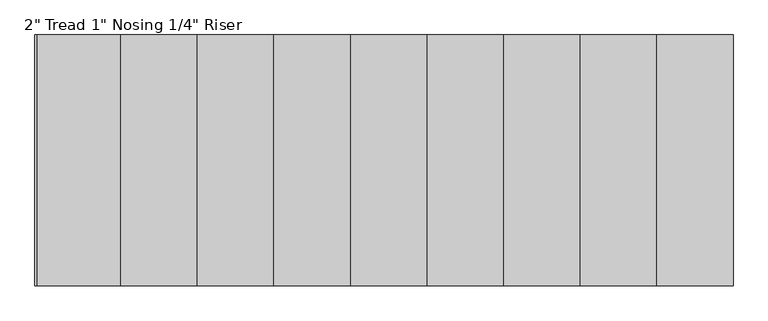
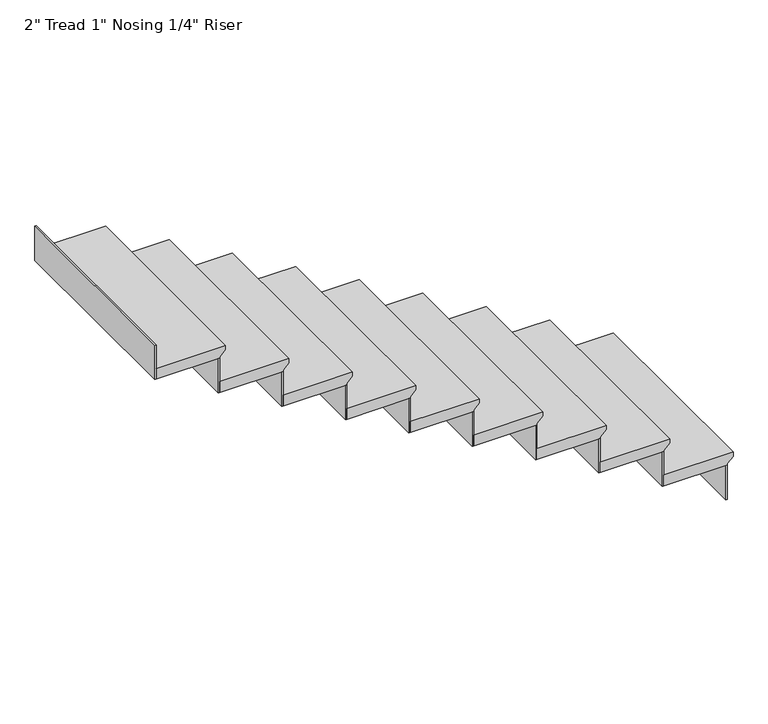
"""IFC4 building model written with IfcOpenShell, lengths in millimetres: stair flight geometry."""

from ifc_helpers import new_model, si_unit, frame, origin, place, context, project, spatial, polyline, outline, extrude, source, transform, mapped, element, save


def stair_flight_043378c7(model_context):
    return source(origin(), model_context, "Body", "SweptSolid", [
        extrude(outline(polyline([(4960.62, 923.4845537), (4960.62, 618.6845537), (4909.82, 618.6845537), (4909.82, 898.0845537), (4916.17, 898.0845537), (4941.57, 923.4845537), (4960.62, 923.4845537)])), frame((0.0, -5753.3544725, 0.0), z_axis=(0.0, 1.0, 0.0), x_axis=(0.0, 0.0, 1.0)), (0.0, 0.0, 1.0), 914.4),
        extrude(outline(polyline([(891.7345537, -4838.9544725), (898.0845537, -4838.9544725), (898.0845537, -5753.3544725), (891.7345537, -5753.3544725), (891.7345537, -4838.9544725)])), frame((0.0, 0.0, 4749.8), z_axis=(0.0, 0.0, 1.0), x_axis=(1.0, 0.0, 0.0)), (0.0, 0.0, 1.0), 160.02),
        extrude(outline(polyline([(612.3345537, -4838.9544725), (618.6845537, -4838.9544725), (618.6845537, -5753.3544725), (612.3345537, -5753.3544725), (612.3345537, -4838.9544725)])), frame((0.0, 0.0, 4909.82), z_axis=(0.0, 0.0, 1.0), x_axis=(1.0, 0.0, 0.0)), (0.0, 0.0, 1.0), 160.02),
        extrude(outline(polyline([(5120.64, 644.0845537), (5120.64, 339.2845537), (5069.84, 339.2845537), (5069.84, 618.6845537), (5076.19, 618.6845537), (5101.59, 644.0845537), (5120.64, 644.0845537)])), frame((0.0, -5753.3544725, 0.0), z_axis=(0.0, 1.0, 0.0), x_axis=(0.0, 0.0, 1.0)), (0.0, 0.0, 1.0), 914.4),
        extrude(outline(polyline([(332.9345537, -4838.9544725), (339.2845537, -4838.9544725), (339.2845537, -5753.3544725), (332.9345537, -5753.3544725), (332.9345537, -4838.9544725)])), frame((0.0, 0.0, 5069.84), z_axis=(0.0, 0.0, 1.0), x_axis=(1.0, 0.0, 0.0)), (0.0, 0.0, 1.0), 160.02),
        extrude(outline(polyline([(5280.66, 364.6845537), (5280.66, 59.8845537), (5229.86, 59.8845537), (5229.86, 339.2845537), (5236.21, 339.2845537), (5261.61, 364.6845537), (5280.66, 364.6845537)])), frame((0.0, -5753.3544725, 0.0), z_axis=(0.0, 1.0, 0.0), x_axis=(0.0, 0.0, 1.0)), (0.0, 0.0, 1.0), 914.4),
        extrude(outline(polyline([(53.5345537, -4838.9544725), (59.8845537, -4838.9544725), (59.8845537, -5753.3544725), (53.5345537, -5753.3544725), (53.5345537, -4838.9544725)])), frame((0.0, 0.0, 5229.86), z_axis=(0.0, 0.0, 1.0), x_axis=(1.0, 0.0, 0.0)), (0.0, 0.0, 1.0), 160.02),
        extrude(outline(polyline([(5440.68, 85.2845537), (5440.68, -219.5154463), (5389.88, -219.5154463), (5389.88, 59.8845537), (5396.23, 59.8845537), (5421.63, 85.2845537), (5440.68, 85.2845537)])), frame((0.0, -5753.3544725, 0.0), z_axis=(0.0, 1.0, 0.0), x_axis=(0.0, 0.0, 1.0)), (0.0, 0.0, 1.0), 914.4),
        extrude(outline(polyline([(-225.8654463, -4838.9544725), (-219.5154463, -4838.9544725), (-219.5154463, -5753.3544725), (-225.8654463, -5753.3544725), (-225.8654463, -4838.9544725)])), frame((0.0, 0.0, 5389.88), z_axis=(0.0, 0.0, 1.0), x_axis=(1.0, 0.0, 0.0)), (0.0, 0.0, 1.0), 160.02),
        extrude(outline(polyline([(5600.7, -194.1154463), (5600.7, -498.9154463), (5549.9, -498.9154463), (5549.9, -219.5154463), (5556.25, -219.5154463), (5581.65, -194.1154463), (5600.7, -194.1154463)])), frame((0.0, -5753.3544725, 0.0), z_axis=(0.0, 1.0, 0.0), x_axis=(0.0, 0.0, 1.0)), (0.0, 0.0, 1.0), 914.4),
        extrude(outline(polyline([(-505.2654463, -4838.9544725), (-498.9154463, -4838.9544725), (-498.9154463, -5753.3544725), (-505.2654463, -5753.3544725), (-505.2654463, -4838.9544725)])), frame((0.0, 0.0, 5549.9), z_axis=(0.0, 0.0, 1.0), x_axis=(1.0, 0.0, 0.0)), (0.0, 0.0, 1.0), 160.02),
        extrude(outline(polyline([(5760.72, -473.5154463), (5760.72, -778.3154463), (5709.92, -778.3154463), (5709.92, -498.9154463), (5716.27, -498.9154463), (5741.67, -473.5154463), (5760.72, -473.5154463)])), frame((0.0, -5753.3544725, 0.0), z_axis=(0.0, 1.0, 0.0), x_axis=(0.0, 0.0, 1.0)), (0.0, 0.0, 1.0), 914.4),
        extrude(outline(polyline([(-784.6654463, -4838.9544725), (-778.3154463, -4838.9544725), (-778.3154463, -5753.3544725), (-784.6654463, -5753.3544725), (-784.6654463, -4838.9544725)])), frame((0.0, 0.0, 5709.92), z_axis=(0.0, 0.0, 1.0), x_axis=(1.0, 0.0, 0.0)), (0.0, 0.0, 1.0), 160.02),
        extrude(outline(polyline([(5920.74, -752.9154463), (5920.74, -1057.7154463), (5869.94, -1057.7154463), (5869.94, -778.3154463), (5876.29, -778.3154463), (5901.69, -752.9154463), (5920.74, -752.9154463)])), frame((0.0, -5753.3544725, 0.0), z_axis=(0.0, 1.0, 0.0), x_axis=(0.0, 0.0, 1.0)), (0.0, 0.0, 1.0), 914.4),
        extrude(outline(polyline([(-1064.0654463, -4838.9544725), (-1057.7154463, -4838.9544725), (-1057.7154463, -5753.3544725), (-1064.0654463, -5753.3544725), (-1064.0654463, -4838.9544725)])), frame((0.0, 0.0, 5869.94), z_axis=(0.0, 0.0, 1.0), x_axis=(1.0, 0.0, 0.0)), (0.0, 0.0, 1.0), 160.02),
        extrude(outline(polyline([(6080.76, -1032.3154463), (6080.76, -1337.1154463), (6029.96, -1337.1154463), (6029.96, -1057.7154463), (6036.31, -1057.7154463), (6061.71, -1032.3154463), (6080.76, -1032.3154463)])), frame((0.0, -5753.3544725, 0.0), z_axis=(0.0, 1.0, 0.0), x_axis=(0.0, 0.0, 1.0)), (0.0, 0.0, 1.0), 914.4),
        extrude(outline(polyline([(-1343.4654463, -4838.9544725), (-1337.1154463, -4838.9544725), (-1337.1154463, -5753.3544725), (-1343.4654463, -5753.3544725), (-1343.4654463, -4838.9544725)])), frame((0.0, 0.0, 6029.96), z_axis=(0.0, 0.0, 1.0), x_axis=(1.0, 0.0, 0.0)), (0.0, 0.0, 1.0), 160.02),
        extrude(outline(polyline([(-1622.8654463, -4838.9544725), (-1616.5154463, -4838.9544725), (-1616.5154463, -5753.3544725), (-1622.8654463, -5753.3544725), (-1622.8654463, -4838.9544725)])), frame((0.0, 0.0, 6189.98), z_axis=(0.0, 0.0, 1.0), x_axis=(1.0, 0.0, 0.0)), (0.0, 0.0, 1.0), 160.02),
        extrude(outline(polyline([(6240.78, -1311.7154463), (6240.78, -1616.5154463), (6189.98, -1616.5154463), (6189.98, -1337.1154463), (6196.33, -1337.1154463), (6221.73, -1311.7154463), (6240.78, -1311.7154463)])), frame((0.0, -5753.3544725, 0.0), z_axis=(0.0, 1.0, 0.0), x_axis=(0.0, 0.0, 1.0)), (0.0, 0.0, 1.0), 914.4),
    ])


if __name__ == "__main__":
    model = new_model("IFC4")
    model_context = context("Model", 3, world=origin())
    ifc_project = project(units=[si_unit("LENGTHUNIT", "METRE", prefix="MILLI")], contexts=[model_context])
    site = spatial("IfcSite", under=ifc_project)
    building = spatial("IfcBuilding", under=site)
    placement = place(None, origin())
    stair_flight_shape = stair_flight_043378c7(model_context)
    element("IfcStairFlight", 1, ObjectType="2\" Tread 1\" Nosing 1/4\" Riser", at=placement, inside=building, context=model_context, shape_type="MappedRepresentation", body=[
        mapped(stair_flight_shape, transform((0.0, 0.0, 0.0), x_axis=(1.0, 0.0, 0.0), y_axis=(0.0, 1.0, 0.0), z_axis=(0.0, 0.0, 1.0))),
    ])
    save(model, "model.ifc")
